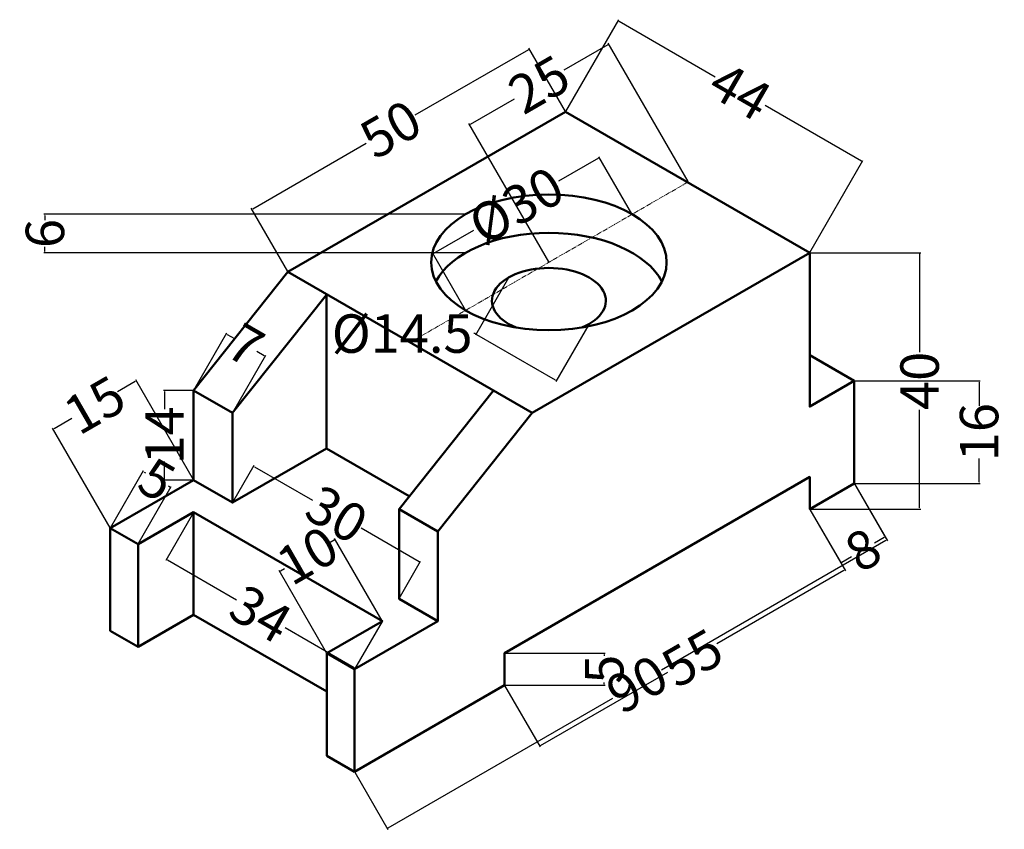
# Model space of a CAD drawing. Units: millimetres. Extents: x -12 to 142, y 32 to 158.
import ezdxf

# ---------------------------------------------------------------- set-up
doc = ezdxf.new("R2010")
doc.units = ezdxf.units.MM
doc.header["$MEASUREMENT"] = 0
doc.linetypes.add('CENTER2', pattern=[1.125, 0.75, -0.125, 0.125, -0.125])
for name, color, linetype, lineweight in [('M-CNTR', 4, 'CENTER2', 18), ('M-DIMS', 2, 'Continuous', 25), ('M-OUTL', 7, 'Continuous', 50)]:
    doc.layers.add(name, color=color, linetype=linetype, lineweight=lineweight)
doc.styles.get("Standard").update_dxf_attribs({"font": 'arial.ttf'})
doc.dimstyles.get("Standard").update_dxf_attribs({"dimtxt": 6, "dimasz": 0.18, "dimexe": 0.18, "dimexo": 0.0625, "dimgap": 0.09, "dimtad": 0, "dimtoh": 1, "dimdec": 0, "dimzin": 0, "dimdsep": 46, "dimtxsty": 'Standard', "dimcen": 0.09, "dimadec": 0, "dimazin": 0, "dimtfac": 1, "dimtdec": 0, "dimtofl": 0, "dimtmove": 0, "dimatfit": 3, "dimfxl": 1, "dimtolj": 1, "dimtzin": 0, "dimarcsym": 0})

# ---------------------------------------------------------------- blocks, each defined once
blk = doc.blocks.new('*D1')
at = {"layer": 'Defpoints', "color": 0, "transparency": 16777216}
for p in [(15.05, 81.51), (44.5, 64.51), (40.25, 57.16)]:
    blk.add_point(p, dxfattribs=at)
at = {"layer": 'M-DIMS', "color": 0, "lineweight": -2, "transparency": 16777216}
for p, q in [((15.02, 81.46), (10.72, 74)), ((10.96, 74.07), (21.74, 67.85)), ((40.1, 57.25), (29.32, 63.47)), ((44.47, 64.46), (40.16, 57))]:
    blk.add_line(p, q, dxfattribs=at)
at = {"layer": 'M-DIMS', "color": 0, "transparency": 16777216}
for points in [[(10.98, 74.09), (10.95, 74.04), (10.81, 74.16)], [(40.11, 57.27), (40.08, 57.22), (40.25, 57.16)]]:
    blk.add_solid(points, dxfattribs=at)
at = {"layer": 'M-DIMS', "color": 0, "transparency": 16777216, "insert": (25.53, 65.66), "char_height": 6, "attachment_point": 5, "rotation": 330}
blk.add_mtext('\\A1;34', dxfattribs=at)
blk = doc.blocks.new('*D2')
at = {"layer": 'Defpoints', "color": 0, "transparency": 16777216}
for p in [(118.11, 86.01), (111.18, 82.01), (122.94, 77.64)]:
    blk.add_point(p, dxfattribs=at)
at = {"layer": 'M-DIMS', "color": 0, "lineweight": -2, "transparency": 16777216}
for p, q in [((118.14, 85.96), (123.03, 77.48)), ((111.21, 81.96), (116.11, 73.48)), ((122.79, 77.55), (121.27, 76.67)), ((116.17, 73.73), (117.69, 74.6))]:
    blk.add_line(p, q, dxfattribs=at)
at = {"layer": 'M-DIMS', "color": 0, "transparency": 16777216}
for points in [[(122.77, 77.57), (122.8, 77.52), (122.94, 77.64)], [(116.16, 73.75), (116.19, 73.7), (116.02, 73.64)]]:
    blk.add_solid(points, dxfattribs=at)
at = {"layer": 'M-DIMS', "color": 0, "transparency": 16777216, "insert": (119.48, 75.64), "char_height": 6, "attachment_point": 5, "rotation": 30}
blk.add_mtext('\\A1;8', dxfattribs=at)
blk = doc.blocks.new('*D3')
at = {"layer": 'Defpoints', "color": 0, "transparency": 16777216}
for p in [(118.11, 102.01), (118.11, 86.01), (137.59, 86.01)]:
    blk.add_point(p, dxfattribs=at)
at = {"layer": 'M-DIMS', "color": 0, "lineweight": -2, "transparency": 16777216}
for p, q in [((118.17, 102.01), (137.77, 102.01)), ((137.59, 101.83), (137.59, 98.12)), ((137.59, 86.19), (137.59, 89.91)), ((118.17, 86.01), (137.77, 86.01))]:
    blk.add_line(p, q, dxfattribs=at)
at = {"layer": 'M-DIMS', "color": 0, "transparency": 16777216}
for points in [[(137.56, 101.83), (137.62, 101.83), (137.59, 102.01)], [(137.56, 86.19), (137.62, 86.19), (137.59, 86.01)]]:
    blk.add_solid(points, dxfattribs=at)
at = {"layer": 'M-DIMS', "color": 0, "transparency": 16777216, "insert": (137.59, 94.01), "char_height": 6, "attachment_point": 5, "rotation": 90}
blk.add_mtext('\\A1;16', dxfattribs=at)
blk = doc.blocks.new('*D4')
at = {"layer": 'Defpoints', "color": 0, "transparency": 16777216}
for p in [(-6.88, 94.5), (15.05, 86.51), (2.06, 79.01)]:
    blk.add_point(p, dxfattribs=at)
at = {"layer": 'M-DIMS', "color": 0, "lineweight": -2, "transparency": 16777216}
for p, q in [((5.96, 101.91), (3.19, 100.31)), ((15.02, 86.57), (6.02, 102.15)), ((-6.72, 94.59), (-3.96, 96.18)), ((2.03, 79.07), (-6.97, 94.65))]:
    blk.add_line(p, q, dxfattribs=at)
at = {"layer": 'M-DIMS', "color": 0, "transparency": 16777216}
for points in [[(5.94, 101.93), (5.97, 101.88), (6.11, 102)], [(-6.74, 94.61), (-6.71, 94.56), (-6.88, 94.5)]]:
    blk.add_solid(points, dxfattribs=at)
at = {"layer": 'M-DIMS', "color": 0, "transparency": 16777216, "insert": (-0.38, 98.25), "char_height": 6, "attachment_point": 5, "rotation": 30}
blk.add_mtext('\\A1;15', dxfattribs=at)
blk = doc.blocks.new('*D5')
at = {"layer": 'Defpoints', "color": 0, "transparency": 16777216}
for p in [(15.05, 100.51), (10.52, 86.51), (15.05, 86.51)]:
    blk.add_point(p, dxfattribs=at)
at = {"layer": 'M-DIMS', "color": 0, "lineweight": -2, "transparency": 16777216}
for p, q in [((14.99, 100.51), (10.34, 100.51)), ((10.52, 100.33), (10.52, 97.6)), ((10.52, 86.69), (10.52, 89.42)), ((14.99, 86.51), (10.34, 86.51))]:
    blk.add_line(p, q, dxfattribs=at)
at = {"layer": 'M-DIMS', "color": 0, "transparency": 16777216}
for points in [[(10.49, 100.33), (10.55, 100.33), (10.52, 100.51)], [(10.49, 86.69), (10.55, 86.69), (10.52, 86.51)]]:
    blk.add_solid(points, dxfattribs=at)
at = {"layer": 'M-DIMS', "color": 0, "transparency": 16777216, "insert": (10.52, 93.51), "char_height": 6, "attachment_point": 5, "rotation": 90}
blk.add_mtext('\\A1;14', dxfattribs=at)
blk = doc.blocks.new('*D6')
at = {"layer": 'Defpoints', "color": 0, "transparency": 16777216}
for p in [(21.12, 83.01), (50.38, 73.7), (47.1, 68.01)]:
    blk.add_point(p, dxfattribs=at)
at = {"layer": 'M-DIMS', "color": 0, "lineweight": -2, "transparency": 16777216}
for p, q in [((21.15, 83.07), (24.49, 88.85)), ((24.55, 88.61), (33.6, 83.39)), ((50.22, 73.79), (41.18, 79.01)), ((47.13, 68.07), (50.47, 73.85))]:
    blk.add_line(p, q, dxfattribs=at)
at = {"layer": 'M-DIMS', "color": 0, "transparency": 16777216}
for points in [[(24.57, 88.63), (24.54, 88.58), (24.4, 88.7)], [(50.24, 73.81), (50.21, 73.76), (50.38, 73.7)]]:
    blk.add_solid(points, dxfattribs=at)
at = {"layer": 'M-DIMS', "color": 0, "transparency": 16777216, "insert": (37.39, 81.2), "char_height": 6, "attachment_point": 5, "rotation": 330}
blk.add_mtext('\\A1;30', dxfattribs=at)
blk = doc.blocks.new('*D7')
at = {"layer": 'Defpoints', "color": 0, "transparency": 16777216}
for p in [(73.08, 144.01), (119.39, 136.22), (111.18, 122.01)]:
    blk.add_point(p, dxfattribs=at)
at = {"layer": 'M-DIMS', "color": 0, "lineweight": -2, "transparency": 16777216}
for p, q in [((73.11, 144.07), (81.37, 158.38)), ((81.44, 158.13), (96.44, 149.47)), ((119.23, 136.31), (104.23, 144.98)), ((111.21, 122.07), (119.48, 136.38))]:
    blk.add_line(p, q, dxfattribs=at)
at = {"layer": 'M-DIMS', "color": 0, "transparency": 16777216}
for points in [[(81.45, 158.16), (81.42, 158.11), (81.28, 158.22)], [(119.25, 136.34), (119.22, 136.29), (119.39, 136.22)]]:
    blk.add_solid(points, dxfattribs=at)
at = {"layer": 'M-DIMS', "color": 0, "transparency": 16777216, "insert": (100.33, 147.22), "char_height": 6, "attachment_point": 5, "rotation": 330}
blk.add_mtext('\\A1;44', dxfattribs=at)
blk = doc.blocks.new('*D8')
at = {"layer": 'Defpoints', "color": 0, "transparency": 16777216}
for p in [(67.44, 153.78), (73.08, 144.01), (29.78, 119.01)]:
    blk.add_point(p, dxfattribs=at)
at = {"layer": 'M-DIMS', "color": 0, "lineweight": -2, "transparency": 16777216}
for p, q in [((67.28, 153.69), (49.58, 143.47)), ((73.05, 144.07), (67.35, 153.94)), ((24.29, 128.87), (41.99, 139.09)), ((29.74, 119.07), (24.05, 128.94))]:
    blk.add_line(p, q, dxfattribs=at)
at = {"layer": 'M-DIMS', "color": 0, "transparency": 16777216}
for points in [[(67.27, 153.72), (67.3, 153.67), (67.44, 153.78)], [(24.28, 128.9), (24.31, 128.85), (24.14, 128.78)]]:
    blk.add_solid(points, dxfattribs=at)
at = {"layer": 'M-DIMS', "color": 0, "transparency": 16777216, "insert": (45.79, 141.28), "char_height": 6, "attachment_point": 5, "rotation": 30}
blk.add_mtext('\\A1;50', dxfattribs=at)
blk = doc.blocks.new('*D9')
at = {"layer": 'Defpoints', "color": 0, "transparency": 16777216}
for p in [(79.83, 154.56), (92.23, 133.07), (70.48, 120.51)]:
    blk.add_point(p, dxfattribs=at)
at = {"layer": 'M-DIMS', "color": 0, "lineweight": -2, "transparency": 16777216}
for p, q in [((79.67, 154.47), (72.81, 150.51)), ((92.2, 133.13), (79.74, 154.72)), ((58.23, 142.09), (65.09, 146.05)), ((70.45, 120.57), (57.98, 142.16))]:
    blk.add_line(p, q, dxfattribs=at)
at = {"layer": 'M-DIMS', "color": 0, "transparency": 16777216}
for points in [[(79.66, 154.5), (79.69, 154.45), (79.83, 154.56)], [(58.21, 142.12), (58.24, 142.07), (58.07, 142)]]:
    blk.add_solid(points, dxfattribs=at)
at = {"layer": 'M-DIMS', "color": 0, "transparency": 16777216, "insert": (68.95, 148.28), "char_height": 6, "attachment_point": 5, "rotation": 30}
blk.add_mtext('\\A1;25', dxfattribs=at)
blk = doc.blocks.new('*D10')
at = {"layer": 'Defpoints', "color": 0, "transparency": 16777216}
for p in [(111.18, 82.01), (116.66, 72.52), (63.55, 54.51)]:
    blk.add_point(p, dxfattribs=at)
at = {"layer": 'M-DIMS', "color": 0, "lineweight": -2, "transparency": 16777216}
for p, q in [((111.21, 81.96), (116.75, 72.37)), ((116.5, 72.43), (96.66, 60.98)), ((69.18, 45.11), (89.02, 56.57)), ((63.58, 54.46), (69.12, 44.87))]:
    blk.add_line(p, q, dxfattribs=at)
at = {"layer": 'M-DIMS', "color": 0, "transparency": 16777216}
for points in [[(116.49, 72.46), (116.52, 72.41), (116.66, 72.52)], [(69.17, 45.14), (69.2, 45.09), (69.03, 45.02)]]:
    blk.add_solid(points, dxfattribs=at)
at = {"layer": 'M-DIMS', "color": 0, "transparency": 16777216, "insert": (92.84, 58.77), "char_height": 6, "attachment_point": 5, "rotation": 30}
blk.add_mtext('\\A1;55', dxfattribs=at)
blk = doc.blocks.new('*D11')
at = {"layer": 'Defpoints', "color": 0, "transparency": 16777216}
for p in [(63.55, 59.51), (63.55, 54.51), (79.1, 54.51)]:
    blk.add_point(p, dxfattribs=at)
at = {"layer": 'M-DIMS', "color": 0, "lineweight": -2, "transparency": 16777216}
for p, q in [((63.61, 59.51), (79.28, 59.51)), ((79.1, 59.33), (79.1, 59.09)), ((63.61, 54.51), (79.28, 54.51)), ((79.1, 54.69), (79.1, 54.93))]:
    blk.add_line(p, q, dxfattribs=at)
at = {"layer": 'M-DIMS', "color": 0, "transparency": 16777216}
for points in [[(79.07, 59.33), (79.13, 59.33), (79.1, 59.51)], [(79.07, 54.69), (79.13, 54.69), (79.1, 54.51)]]:
    blk.add_solid(points, dxfattribs=at)
at = {"layer": 'M-DIMS', "color": 0, "transparency": 16777216, "insert": (79.1, 57.01), "char_height": 6, "attachment_point": 5, "rotation": 90}
blk.add_mtext('\\A1;5', dxfattribs=at)
blk = doc.blocks.new('*D12')
at = {"layer": 'Defpoints', "color": 0, "transparency": 16777216}
for p in [(37.14, 77.26), (44.5, 64.51), (35.84, 59.51)]:
    blk.add_point(p, dxfattribs=at)
at = {"layer": 'M-DIMS', "color": 0, "lineweight": -2, "transparency": 16777216}
for p, q in [((36.98, 77.17), (36.35, 76.81)), ((44.47, 64.57), (37.05, 77.42)), ((35.81, 59.57), (28.39, 72.42)), ((28.63, 72.35), (29.26, 72.71))]:
    blk.add_line(p, q, dxfattribs=at)
at = {"layer": 'M-DIMS', "color": 0, "transparency": 16777216}
for points in [[(36.97, 77.2), (37, 77.15), (37.14, 77.26)], [(28.62, 72.38), (28.65, 72.33), (28.48, 72.26)]]:
    blk.add_solid(points, dxfattribs=at)
at = {"layer": 'M-DIMS', "color": 0, "transparency": 16777216, "insert": (32.81, 74.76), "char_height": 6, "attachment_point": 5, "rotation": 30}
blk.add_mtext('\\A1;10', dxfattribs=at)
blk = doc.blocks.new('*D13')
at = {"layer": 'Defpoints', "color": 0, "transparency": 16777216}
for p in [(118.11, 86.01), (40.17, 41.01), (45.27, 32.18)]:
    blk.add_point(p, dxfattribs=at)
at = {"layer": 'M-DIMS', "color": 0, "lineweight": -2, "transparency": 16777216}
for p, q in [((118.14, 85.96), (123.3, 77.02)), ((123.05, 77.09), (88.03, 56.87)), ((45.42, 32.27), (80.45, 52.49)), ((40.2, 40.96), (45.36, 32.02))]:
    blk.add_line(p, q, dxfattribs=at)
at = {"layer": 'M-DIMS', "color": 0, "transparency": 16777216}
for points in [[(123.04, 77.11), (123.07, 77.06), (123.21, 77.18)], [(45.41, 32.29), (45.44, 32.24), (45.27, 32.18)]]:
    blk.add_solid(points, dxfattribs=at)
at = {"layer": 'M-DIMS', "color": 0, "transparency": 16777216, "insert": (84.24, 54.68), "char_height": 6, "attachment_point": 5, "rotation": 30}
blk.add_mtext('\\A1;90', dxfattribs=at)
blk = doc.blocks.new('*D14')
at = {"layer": 'Defpoints', "color": 0, "transparency": 16777216}
for p in [(111.18, 122.01), (128.31, 122.01), (111.18, 82.01)]:
    blk.add_point(p, dxfattribs=at)
at = {"layer": 'M-DIMS', "color": 0, "lineweight": -2, "transparency": 16777216}
for p, q in [((111.24, 122.01), (128.49, 122.01)), ((128.31, 121.83), (128.31, 106.51)), ((128.31, 82.19), (128.31, 97.51)), ((111.24, 82.01), (128.49, 82.01))]:
    blk.add_line(p, q, dxfattribs=at)
at = {"layer": 'M-DIMS', "color": 0, "transparency": 16777216}
for points in [[(128.28, 121.83), (128.34, 121.83), (128.31, 122.01)], [(128.28, 82.19), (128.34, 82.19), (128.31, 82.01)]]:
    blk.add_solid(points, dxfattribs=at)
at = {"layer": 'M-DIMS', "color": 0, "transparency": 16777216, "insert": (128.31, 102.01), "char_height": 6, "attachment_point": 5, "rotation": 90}
blk.add_mtext('\\A1;40', dxfattribs=at)
blk = doc.blocks.new('*D15')
at = {"layer": 'Defpoints', "color": 0, "transparency": 16777216}
for p in [(78.37, 136.85), (83.47, 128.01), (57.49, 113.01)]:
    blk.add_point(p, dxfattribs=at)
at = {"layer": 'M-DIMS', "color": 0, "lineweight": -2, "transparency": 16777216}
for p, q in [((78.21, 136.76), (72, 133.17)), ((83.44, 128.07), (78.28, 137)), ((52.54, 121.94), (58.76, 125.53)), ((57.46, 113.07), (52.3, 122))]:
    blk.add_line(p, q, dxfattribs=at)
at = {"layer": 'M-DIMS', "color": 0, "transparency": 16777216}
for points in [[(78.2, 136.78), (78.23, 136.73), (78.37, 136.85)], [(52.53, 121.96), (52.56, 121.91), (52.39, 121.85)]]:
    blk.add_solid(points, dxfattribs=at)
at = {"layer": 'M-DIMS', "color": 0, "transparency": 16777216, "insert": (65.38, 129.35), "char_height": 6, "attachment_point": 5, "rotation": 30}
blk.add_mtext('\\A1;%%c30', dxfattribs=at)
blk = doc.blocks.new('*D16')
at = {"layer": 'Defpoints', "color": 0, "transparency": 16777216}
for p in [(64.2, 118.14), (76.76, 110.89), (59.1, 109.3)]:
    blk.add_point(p, dxfattribs=at)
at = {"layer": 'M-DIMS', "color": 0, "lineweight": -2, "transparency": 16777216}
for p, q in [((64.17, 118.08), (59.01, 109.15)), ((76.73, 110.83), (71.57, 101.9)), ((58.94, 109.39), (58.76, 109.39)), ((59.1, 109.3), (58.94, 109.39)), ((71.5, 102.14), (59.26, 109.21))]:
    blk.add_line(p, q, dxfattribs=at)
at = {"layer": 'M-DIMS', "color": 0, "transparency": 16777216}
for points in [[(59.27, 109.24), (59.24, 109.19), (59.1, 109.3)], [(71.52, 102.17), (71.49, 102.12), (71.66, 102.05)]]:
    blk.add_solid(points, dxfattribs=at)
at = {"layer": 'M-DIMS', "color": 0, "transparency": 16777216, "insert": (47.59, 109.39), "char_height": 6, "attachment_point": 5}
blk.add_mtext('\\A1;%%c14.5', dxfattribs=at)
blk = doc.blocks.new('*D17')
at = {"layer": 'Defpoints', "color": 0, "transparency": 16777216}
for p in [(57.49, 128.01), (-8.14, 122.01), (57.49, 122.01)]:
    blk.add_point(p, dxfattribs=at)
at = {"layer": 'M-DIMS', "color": 0, "lineweight": -2, "transparency": 16777216}
for p, q in [((57.43, 128.01), (-8.32, 128.01)), ((-8.14, 127.83), (-8.14, 127.08)), ((-8.14, 122.19), (-8.14, 122.94)), ((57.43, 122.01), (-8.32, 122.01))]:
    blk.add_line(p, q, dxfattribs=at)
at = {"layer": 'M-DIMS', "color": 0, "transparency": 16777216}
for points in [[(-8.17, 127.83), (-8.11, 127.83), (-8.14, 128.01)], [(-8.17, 122.19), (-8.11, 122.19), (-8.14, 122.01)]]:
    blk.add_solid(points, dxfattribs=at)
at = {"layer": 'M-DIMS', "color": 0, "transparency": 16777216, "insert": (-8.14, 125.01), "char_height": 6, "attachment_point": 5, "rotation": 90}
blk.add_mtext('\\A1;6', dxfattribs=at)
blk = doc.blocks.new('*D18')
at = {"layer": 'Defpoints', "color": 0, "transparency": 16777216}
for p in [(26.22, 105.85), (15.05, 100.51), (21.12, 97.01)]:
    blk.add_point(p, dxfattribs=at)
at = {"layer": 'M-DIMS', "color": 0, "lineweight": -2, "transparency": 16777216}
for p, q in [((15.08, 100.57), (20.24, 109.5)), ((20.31, 109.26), (21.42, 108.61)), ((21.15, 97.07), (26.31, 106)), ((26.06, 105.94), (24.94, 106.58))]:
    blk.add_line(p, q, dxfattribs=at)
at = {"layer": 'M-DIMS', "color": 0, "transparency": 16777216}
for points in [[(20.32, 109.28), (20.29, 109.23), (20.15, 109.35)], [(26.07, 105.96), (26.04, 105.91), (26.22, 105.85)]]:
    blk.add_solid(points, dxfattribs=at)
at = {"layer": 'M-DIMS', "color": 0, "transparency": 16777216, "insert": (23.18, 107.6), "char_height": 6, "attachment_point": 5, "rotation": 330}
blk.add_mtext('\\A1;7', dxfattribs=at)
blk = doc.blocks.new('*D19')
at = {"layer": 'Defpoints', "color": 0, "transparency": 16777216}
for p in [(11.49, 85.35), (2.06, 79.01), (6.39, 76.51)]:
    blk.add_point(p, dxfattribs=at)
at = {"layer": 'M-DIMS', "color": 0, "lineweight": -2, "transparency": 16777216}
for p, q in [((2.09, 79.07), (7.25, 88)), ((7.32, 87.76), (7.53, 87.64)), ((6.42, 76.57), (11.58, 85.5)), ((11.34, 85.44), (11.13, 85.56))]:
    blk.add_line(p, q, dxfattribs=at)
at = {"layer": 'M-DIMS', "color": 0, "transparency": 16777216}
for points in [[(7.33, 87.78), (7.3, 87.73), (7.16, 87.85)], [(11.35, 85.46), (11.32, 85.41), (11.49, 85.35)]]:
    blk.add_solid(points, dxfattribs=at)
at = {"layer": 'M-DIMS', "color": 0, "transparency": 16777216, "insert": (9.33, 86.6), "char_height": 6, "attachment_point": 5, "rotation": 330}
blk.add_mtext('\\A1;5', dxfattribs=at)

msp = doc.modelspace()

# ---------------------------------------------------------------- linework, layer by layer
at = {"layer": 'M-CNTR'}
msp.add_line((48.72, 107.95), (92.23, 133.07), dxfattribs=at)
at = {"layer": 'M-OUTL'}
msp.add_line((15.05, 65.51), (35.84, 53.51), dxfattribs=at)
for points in [[(48.68, 84.01), (35.8, 91.45), (21.12, 83.01), (21.12, 97.01), (15.05, 100.51), (29.78, 119.01), (73.08, 144.01), (111.18, 122.01), (67.88, 97.01)], [(111.18, 106.01), (118.11, 102.01), (111.18, 98.01), (111.18, 122.01)], [(29.78, 119.01), (67.88, 97.01), (53.16, 78.51), (47.1, 82.01), (61.82, 100.51)], [(21.08, 96.95), (35.8, 115.45), (35.8, 91.45)], [(118.11, 102.01), (118.11, 86.01), (111.18, 82.01), (111.18, 87.01), (111.18, 87.01), (63.55, 59.51), (63.55, 54.51), (40.17, 41.01)], [(21.12, 83.01), (15.05, 86.51), (15.05, 100.51)], [(15.05, 81.51), (6.39, 76.51), (2.06, 79.01), (15.05, 86.51)], [(6.39, 76.51), (6.39, 60.51), (15.05, 65.51), (15.05, 81.51), (44.5, 64.51), (35.84, 59.51), (40.17, 57.01), (53.16, 64.51)], [(53.16, 78.51), (53.16, 64.51), (47.1, 68.01), (47.1, 82.01)], [(6.39, 60.51), (2.06, 63.01), (2.06, 79.01)], [(35.84, 59.51), (35.84, 43.51), (40.17, 41.01), (40.17, 57.01)]]:
    msp.add_lwpolyline(points, dxfattribs=at)
msp.add_ellipse((70.48, 120.51), major_axis=(-18.37, 0), ratio=0.57735, dxfattribs=at)
for major_axis, start_param, end_param in [((-18.37, 0), 3.428349, 5.996429), ((-8.88, 0), 2.186578, 7.2382)]:
    msp.add_ellipse((70.48, 114.51), major_axis=major_axis, ratio=0.57735, start_param=start_param, end_param=end_param, dxfattribs=at)

# ---------------------------------------------------------------- dimensions: what is measured, and where the dimension line sits
at = {"layer": 'M-DIMS'}
for p1, p2, distance, picture, middle in [((73.08, 144.01), (111.18, 122.01), 16.41, '*D7', (100.33, 147.22)), ((29.78, 119.01), (73.08, 144.01), 11.28, '*D8', (45.79, 141.28)), ((70.48, 120.51), (92.23, 133.07), 24.81, '*D9', (68.95, 148.28)), ((15.05, 86.51), (2.06, 79.01), -17.88, '*D4', (-0.38, 98.25)), ((118.11, 102.01), (118.11, 86.01), 19.48, '*D3', (137.59, 94.01)), ((15.05, 100.51), (15.05, 86.51), -4.53, '*D5', (10.52, 93.51)), ((21.12, 83.01), (47.1, 68.01), 6.57, '*D6', (37.39, 81.2)), ((111.18, 82.01), (118.11, 86.01), -9.67, '*D2', (119.48, 75.64)), ((15.05, 81.51), (44.5, 64.51), -8.49, '*D1', (25.53, 65.66)), ((63.55, 54.51), (111.18, 82.01), -10.96, '*D10', (92.84, 58.77)), ((35.84, 59.51), (44.5, 64.51), 14.72, '*D12', (32.81, 74.76)), ((63.55, 59.51), (63.55, 54.51), 15.55, '*D11', (79.1, 57.01))]:
    dim = msp.add_aligned_dim(p1=p1, p2=p2, distance=distance, dimstyle='Standard', override={"dimclrd": 0, "dimclre": 0, "dimclrt": 0}, dxfattribs=at)
    dim.commit()
    dim.dimension.update_dxf_attribs({"geometry": picture, "text_midpoint": middle})
for base, p1, p2, angle, override, picture, middle in [((78.37, 136.85), (57.49, 113.01), (83.47, 128.01), 30, {"dimdec": 0, "dimlfac": 1, "dimrnd": 0, "dimzin": 0, "dimdsep": 46, "dimlunit": 2}, '*D15', (65.38, 129.35)), ((59.1, 109.3), (76.76, 110.89), (64.2, 118.14), 150, {"dimdec": 1, "dimlfac": 1, "dimrnd": 0, "dimzin": 0, "dimdsep": 46, "dimlunit": 2}, '*D16', (47.59, 109.39))]:
    dim = msp.add_linear_dim(base=base, p1=p1, p2=p2, angle=angle, text='%%c<>', dimstyle='Standard', override=override, dxfattribs=at)
    dim.commit()
    dim.dimension.update_dxf_attribs({"geometry": picture, "text_midpoint": middle})
for base, p1, p2, angle, picture, middle in [((-8.14, 122.01), (57.49, 128.01), (57.49, 122.01), 90, '*D17', (-8.14, 125.01)), ((128.31, 122.01), (111.18, 82.01), (111.18, 122.01), 90, '*D14', (128.31, 102.01)), ((26.22, 105.85), (15.05, 100.51), (21.12, 97.01), 330, '*D18', (23.18, 107.6)), ((11.49, 85.35), (2.06, 79.01), (6.39, 76.51), 330, '*D19', (9.33, 86.6)), ((45.27, 32.18), (118.11, 86.01), (40.17, 41.01), 210, '*D13', (84.24, 54.68))]:
    dim = msp.add_linear_dim(base=base, p1=p1, p2=p2, angle=angle, dimstyle='Standard', override={"dimdec": 0, "dimlfac": 1, "dimrnd": 0, "dimzin": 0, "dimdsep": 46, "dimlunit": 2}, dxfattribs=at)
    dim.commit()
    dim.dimension.update_dxf_attribs({"geometry": picture, "text_midpoint": middle})

doc.saveas('drawing.dxf')
